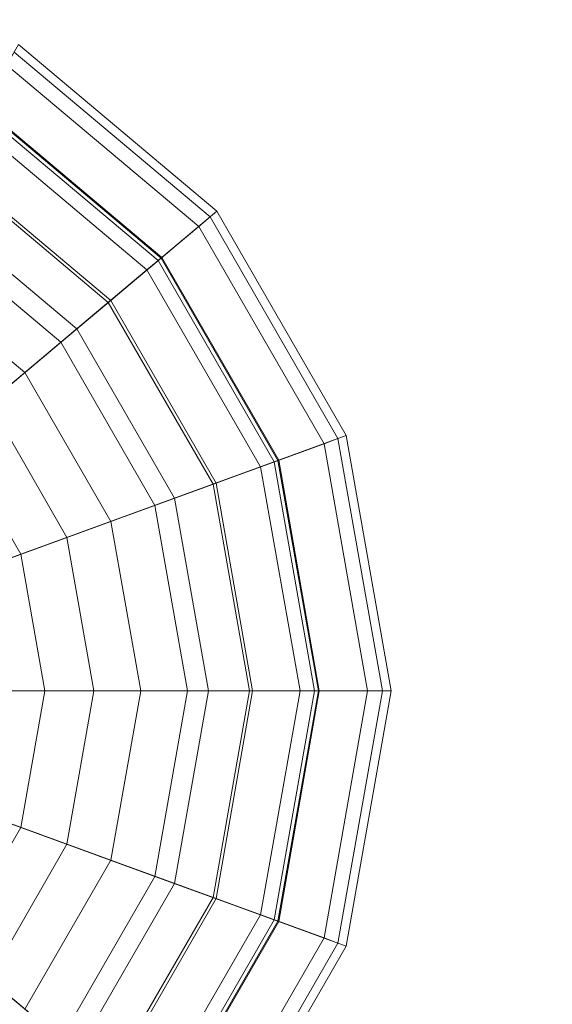
# Model space of a CAD drawing. Units: inches. Extents: x 375 to 1122, y 27 to 1069.
# Tile 100 of 155: x 719.942 to 720.91, y 864.699 to 866.486. Entities that reach past the tile are written whole.
import ezdxf

# ---------------------------------------------------------------- set-up
doc = ezdxf.new("R2010")
doc.units = ezdxf.units.IN
doc.layers.add('A-ANNO-DIMS', color=2, linetype='Continuous', lineweight=18)
doc.layers.add('Furniture', color=30, linetype='Continuous', lineweight=18)
doc.styles.get("Standard").update_dxf_attribs({"font": 'arial.ttf'})
doc.dimstyles.new('ISO-25', dxfattribs={"dimtxt": 12, "dimasz": 2.5, "dimexe": 1.5, "dimexo": 1.5, "dimtad": 1, "dimdec": 1, "dimlunit": 3, "dimtxsty": 'Standard', "dimblk": 'ARCHTICK', "dimcen": 2.5, "dimadec": 0, "dimazin": 0, "dimtfac": 1, "dimtdec": 1, "dimtmove": 0, "dimatfit": 3, "dimfxl": 1.5, "dimfxlon": 1, "dimarcsym": 0})

# ---------------------------------------------------------------- blocks, each defined once
blk = doc.blocks.new('A$C403C54AD')
for points in [[(1.826559, 0.891746, -0.031825), (1.826559, 0.857884, -0.028747), (1.826559, 0.857884, -0.028747), (1.814977, 0.889704, -0.031825)], [(1.826559, 0.88848, -0.028594), (1.826559, 0.891746, -0.031825), (1.814977, 0.889704, -0.031825), (1.816094, 0.886635, -0.028594)], [(1.83814, 0.889704, -0.031825), (1.826559, 0.857884, -0.028747), (1.826559, 0.857884, -0.028747), (1.826559, 0.891746, -0.031825)], [(1.837023, 0.886635, -0.028594), (1.83814, 0.889704, -0.031825), (1.826559, 0.891746, -0.031825), (1.826559, 0.88848, -0.028594)], [(1.826559, 0.88844, 0.131159), (1.826559, 0.891347, 0.117935), (1.815114, 0.889329, 0.117935), (1.816108, 0.886597, 0.131159)], [(1.826559, 0.891347, 0.117935), (1.826559, 0.890672, 0.089693), (1.815345, 0.888695, 0.089693), (1.815114, 0.889329, 0.117935)], [(1.83701, 0.886597, 0.131159), (1.838004, 0.889329, 0.117935), (1.826559, 0.891347, 0.117935), (1.826559, 0.88844, 0.131159)], [(1.838004, 0.889329, 0.117935), (1.837773, 0.888695, 0.089693), (1.826559, 0.890672, 0.089693), (1.826559, 0.891347, 0.117935)], [(1.826559, 0.890672, 0.089693), (1.826559, 0.885308, 0.071684), (1.817179, 0.883654, 0.071684), (1.815345, 0.888695, 0.089693)], [(1.837773, 0.888695, 0.089693), (1.835938, 0.883654, 0.071684), (1.826559, 0.885308, 0.071684), (1.826559, 0.890672, 0.089693)], [(1.816094, 0.886635, -0.028594), (1.814977, 0.889704, -0.031825), (1.804793, 0.883824, -0.031825), (1.806892, 0.881322, -0.028594)], [(1.814977, 0.889704, -0.031825), (1.826559, 0.857884, -0.028747), (1.826559, 0.857884, -0.028747), (1.804793, 0.883824, -0.031825)], [(1.848325, 0.883824, -0.031825), (1.826559, 0.857884, -0.028747), (1.826559, 0.857884, -0.028747), (1.83814, 0.889704, -0.031825)], [(1.846226, 0.881322, -0.028594), (1.848325, 0.883824, -0.031825), (1.83814, 0.889704, -0.031825), (1.837023, 0.886635, -0.028594)], [(1.816108, 0.886597, 0.131159), (1.815114, 0.889329, 0.117935), (1.805049, 0.883518, 0.117935), (1.806918, 0.881291, 0.131159)], [(1.815114, 0.889329, 0.117935), (1.815345, 0.888695, 0.089693), (1.805483, 0.883001, 0.089693), (1.805049, 0.883518, 0.117935)], [(1.8462, 0.881291, 0.131159), (1.848069, 0.883518, 0.117935), (1.838004, 0.889329, 0.117935), (1.83701, 0.886597, 0.131159)], [(1.848069, 0.883518, 0.117935), (1.847635, 0.883001, 0.089693), (1.837773, 0.888695, 0.089693), (1.838004, 0.889329, 0.117935)], [(1.815345, 0.888695, 0.089693), (1.817179, 0.883654, 0.071684), (1.808931, 0.878892, 0.071684), (1.805483, 0.883001, 0.089693)], [(1.826559, 0.872098, -0.02532), (1.826559, 0.88848, -0.028594), (1.816094, 0.886635, -0.028594), (1.821697, 0.871241, -0.02532)], [(1.826559, 0.883444, 0.140564), (1.826559, 0.88844, 0.131159), (1.816108, 0.886597, 0.131159), (1.817817, 0.881902, 0.140564)], [(1.83142, 0.871241, -0.02532), (1.837023, 0.886635, -0.028594), (1.826559, 0.88848, -0.028594), (1.826559, 0.872098, -0.02532)], [(1.835301, 0.881902, 0.140564), (1.83701, 0.886597, 0.131159), (1.826559, 0.88844, 0.131159), (1.826559, 0.883444, 0.140564)], [(1.847635, 0.883001, 0.089693), (1.844187, 0.878892, 0.071684), (1.835938, 0.883654, 0.071684), (1.837773, 0.888695, 0.089693)], [(1.826559, 0.888263, 0.117718), (1.826559, 0.885453, 0.130354), (1.81713, 0.88379, 0.130354), (1.816169, 0.886431, 0.117718)], [(1.826559, 0.887605, 0.090178), (1.826559, 0.888263, 0.117718), (1.816169, 0.886431, 0.117718), (1.816394, 0.885812, 0.090178)], [(1.836949, 0.886431, 0.117718), (1.835988, 0.88379, 0.130354), (1.826559, 0.885453, 0.130354), (1.826559, 0.888263, 0.117718)], [(1.836724, 0.885812, 0.090178), (1.836949, 0.886431, 0.117718), (1.826559, 0.888263, 0.117718), (1.826559, 0.887605, 0.090178)], [(1.826559, 0.882497, 0.073031), (1.826559, 0.887605, 0.090178), (1.816394, 0.885812, 0.090178), (1.818141, 0.881013, 0.073031)], [(1.834977, 0.881013, 0.073031), (1.836724, 0.885812, 0.090178), (1.826559, 0.887605, 0.090178), (1.826559, 0.882497, 0.073031)], [(1.821697, 0.871241, -0.02532), (1.816094, 0.886635, -0.028594), (1.806892, 0.881322, -0.028594), (1.817422, 0.868773, -0.02532)], [(1.817817, 0.881902, 0.140564), (1.816108, 0.886597, 0.131159), (1.806918, 0.881291, 0.131159), (1.81013, 0.877464, 0.140564)], [(1.835696, 0.868773, -0.02532), (1.846226, 0.881322, -0.028594), (1.837023, 0.886635, -0.028594), (1.83142, 0.871241, -0.02532)], [(1.842988, 0.877464, 0.140564), (1.8462, 0.881291, 0.131159), (1.83701, 0.886597, 0.131159), (1.835301, 0.881902, 0.140564)], [(1.816169, 0.886431, 0.117718), (1.81713, 0.88379, 0.130354), (1.808838, 0.879003, 0.130354), (1.807032, 0.881156, 0.117718)], [(1.816394, 0.885812, 0.090178), (1.816169, 0.886431, 0.117718), (1.807032, 0.881156, 0.117718), (1.807455, 0.880651, 0.090178)], [(1.846086, 0.881156, 0.117718), (1.84428, 0.879003, 0.130354), (1.835988, 0.88379, 0.130354), (1.836949, 0.886431, 0.117718)], [(1.845663, 0.880651, 0.090178), (1.846086, 0.881156, 0.117718), (1.836949, 0.886431, 0.117718), (1.836724, 0.885812, 0.090178)], [(1.818141, 0.881013, 0.073031), (1.816394, 0.885812, 0.090178), (1.807455, 0.880651, 0.090178), (1.810738, 0.876739, 0.073031)], [(1.84238, 0.876739, 0.073031), (1.845663, 0.880651, 0.090178), (1.836724, 0.885812, 0.090178), (1.834977, 0.881013, 0.073031)], [(1.826559, 0.885453, 0.130354), (1.826559, 0.880365, 0.140564), (1.81887, 0.879009, 0.140564), (1.81713, 0.88379, 0.130354)], [(1.826559, 0.885308, 0.071684), (1.826559, 0.878242, 0.061451), (1.819596, 0.877014, 0.061451), (1.817179, 0.883654, 0.071684)], [(1.835988, 0.88379, 0.130354), (1.834248, 0.879009, 0.140564), (1.826559, 0.880365, 0.140564), (1.826559, 0.885453, 0.130354)], [(1.835938, 0.883654, 0.071684), (1.833522, 0.877014, 0.061451), (1.826559, 0.878242, 0.061451), (1.826559, 0.885308, 0.071684)], [(1.806892, 0.881322, -0.028594), (1.804793, 0.883824, -0.031825), (1.797233, 0.874815, -0.031825), (1.800062, 0.873182, -0.028594)], [(1.804793, 0.883824, -0.031825), (1.826559, 0.857884, -0.028747), (1.826559, 0.857884, -0.028747), (1.797233, 0.874815, -0.031825)], [(1.855884, 0.874815, -0.031825), (1.826559, 0.857884, -0.028747), (1.826559, 0.857884, -0.028747), (1.848325, 0.883824, -0.031825)], [(1.806918, 0.881291, 0.131159), (1.805049, 0.883518, 0.117935), (1.797579, 0.874616, 0.117935), (1.800097, 0.873162, 0.131159)], [(1.805049, 0.883518, 0.117935), (1.805483, 0.883001, 0.089693), (1.798163, 0.874278, 0.089693), (1.797579, 0.874616, 0.117935)], [(1.81713, 0.88379, 0.130354), (1.81887, 0.879009, 0.140564), (1.812108, 0.875106, 0.140564), (1.808838, 0.879003, 0.130354)], [(1.817179, 0.883654, 0.071684), (1.819596, 0.877014, 0.061451), (1.813473, 0.873479, 0.061451), (1.808931, 0.878892, 0.071684)], [(1.826559, 0.880365, 0.140564), (1.826559, 0.883444, 0.140564), (1.817817, 0.881902, 0.140564), (1.81887, 0.879009, 0.140564)], [(1.834248, 0.879009, 0.140564), (1.835301, 0.881902, 0.140564), (1.826559, 0.883444, 0.140564), (1.826559, 0.880365, 0.140564)], [(1.844187, 0.878892, 0.071684), (1.839644, 0.873479, 0.061451), (1.833522, 0.877014, 0.061451), (1.835938, 0.883654, 0.071684)], [(1.84428, 0.879003, 0.130354), (1.84101, 0.875106, 0.140564), (1.834248, 0.879009, 0.140564), (1.835988, 0.88379, 0.130354)], [(1.805483, 0.883001, 0.089693), (1.808931, 0.878892, 0.071684), (1.802809, 0.871596, 0.071684), (1.798163, 0.874278, 0.089693)], [(1.826559, 0.876011, 0.063639), (1.826559, 0.882497, 0.073031), (1.818141, 0.881013, 0.073031), (1.820359, 0.874918, 0.063639)], [(1.832759, 0.874918, 0.063639), (1.834977, 0.881013, 0.073031), (1.826559, 0.882497, 0.073031), (1.826559, 0.876011, 0.063639)], [(1.81887, 0.879009, 0.140564), (1.817817, 0.881902, 0.140564), (1.81013, 0.877464, 0.140564), (1.812108, 0.875106, 0.140564)], [(1.84101, 0.875106, 0.140564), (1.842988, 0.877464, 0.140564), (1.835301, 0.881902, 0.140564), (1.834248, 0.879009, 0.140564)], [(1.817422, 0.868773, -0.02532), (1.806892, 0.881322, -0.028594), (1.800062, 0.873182, -0.028594), (1.814249, 0.864991, -0.02532)], [(1.81013, 0.877464, 0.140564), (1.806918, 0.881291, 0.131159), (1.800097, 0.873162, 0.131159), (1.804424, 0.870664, 0.140564)], [(1.807032, 0.881156, 0.117718), (1.808838, 0.879003, 0.130354), (1.802683, 0.871669, 0.130354), (1.80025, 0.873073, 0.117718)], [(1.807455, 0.880651, 0.090178), (1.807032, 0.881156, 0.117718), (1.80025, 0.873073, 0.117718), (1.80082, 0.872744, 0.090178)], [(1.838869, 0.864991, -0.02532), (1.853056, 0.873182, -0.028594), (1.846226, 0.881322, -0.028594), (1.835696, 0.868773, -0.02532)], [(1.820359, 0.874918, 0.063639), (1.818141, 0.881013, 0.073031), (1.810738, 0.876739, 0.073031), (1.814907, 0.87177, 0.063639)], [(1.838211, 0.87177, 0.063639), (1.84238, 0.876739, 0.073031), (1.834977, 0.881013, 0.073031), (1.832759, 0.874918, 0.063639)], [(1.810738, 0.876739, 0.073031), (1.807455, 0.880651, 0.090178), (1.80082, 0.872744, 0.090178), (1.805243, 0.87019, 0.073031)], [(1.808838, 0.879003, 0.130354), (1.812108, 0.875106, 0.140564), (1.80709, 0.869125, 0.140564), (1.802683, 0.871669, 0.130354)], [(1.808931, 0.878892, 0.071684), (1.813473, 0.873479, 0.061451), (1.808929, 0.868063, 0.061451), (1.802809, 0.871596, 0.071684)], [(1.850309, 0.871596, 0.071684), (1.844189, 0.868063, 0.061451), (1.839644, 0.873479, 0.061451), (1.844187, 0.878892, 0.071684)], [(1.826559, 0.878242, 0.061451), (1.826559, 0.868003, 0.054084), (1.823098, 0.867392, 0.054084), (1.819596, 0.877014, 0.061451)], [(1.833522, 0.877014, 0.061451), (1.83002, 0.867392, 0.054084), (1.826559, 0.868003, 0.054084), (1.826559, 0.878242, 0.061451)], [(1.812108, 0.875106, 0.140564), (1.81013, 0.877464, 0.140564), (1.804424, 0.870664, 0.140564), (1.80709, 0.869125, 0.140564)], [(1.814907, 0.87177, 0.063639), (1.810738, 0.876739, 0.073031), (1.805243, 0.87019, 0.073031), (1.81086, 0.866948, 0.063639)], [(1.819596, 0.877014, 0.061451), (1.823098, 0.867392, 0.054084), (1.820055, 0.865635, 0.054084), (1.813473, 0.873479, 0.061451)], [(1.839644, 0.873479, 0.061451), (1.833063, 0.865635, 0.054084), (1.83002, 0.867392, 0.054084), (1.833522, 0.877014, 0.061451)], [(1.842258, 0.866948, 0.063639), (1.847874, 0.87019, 0.073031), (1.84238, 0.876739, 0.073031), (1.838211, 0.87177, 0.063639)], [(1.826559, 0.866788, 0.057003), (1.826559, 0.876011, 0.063639), (1.820359, 0.874918, 0.063639), (1.823514, 0.866251, 0.057003)], [(1.829604, 0.866251, 0.057003), (1.832759, 0.874918, 0.063639), (1.826559, 0.876011, 0.063639), (1.826559, 0.866788, 0.057003)], [(1.823514, 0.866251, 0.057003), (1.820359, 0.874918, 0.063639), (1.814907, 0.87177, 0.063639), (1.820835, 0.864705, 0.057003)], [(1.832282, 0.864705, 0.057003), (1.838211, 0.87177, 0.063639), (1.832759, 0.874918, 0.063639), (1.829604, 0.866251, 0.057003)]]:
    blk.add_3dface(points)
blk = doc.blocks.new('_ArchTick')
at = {"color": 0, "linetype": 'ByBlock', "const_width": 0.15}
blk.add_lwpolyline([(-0.5, -0.5), (0.5, 0.5)], dxfattribs=at)
blk = doc.blocks.new('*D85')
at = {"layer": 'A-ANNO-DIMS', "color": 0, "lineweight": -2, "transparency": 16777216}
for p, q in [((401.5073, 868.5277), (398.5073, 868.5277)), ((400.0073, 814.5277), (400.0073, 868.5277)), ((401.5073, 814.5277), (398.5073, 814.5277))]:
    blk.add_line(p, q, dxfattribs=at)
at = {"layer": 'Defpoints', "color": 0, "transparency": 16777216}
for p in [(400.0073, 868.5277), (845.0073, 868.5277), (845.0073, 814.5277)]:
    blk.add_point(p, dxfattribs=at)
at = {"layer": 'A-ANNO-DIMS', "color": 0, "lineweight": -2, "transparency": 16777216, "xscale": 2.5, "yscale": 2.5, "zscale": 2.5}
for p, rotation in [((400.0073, 868.5277), 90), ((400.0073, 814.5277), 270)]:
    blk.add_blockref('_ArchTick', p, dxfattribs=dict(at, rotation=rotation))
at = {"layer": 'A-ANNO-DIMS', "color": 0, "transparency": 16777216, "insert": (393.2555, 841.5277), "char_height": 12, "attachment_point": 5, "rotation": 90}
blk.add_mtext('4\'-6"', dxfattribs=at)

msp = doc.modelspace()

# ---------------------------------------------------------------- block references
at = {"layer": 'Furniture', "xscale": 39.9918517141215, "yscale": 39.9918517141215, "zscale": 39.9918517141215, "rotation": 270}
msp.add_blockref('A$C403C54AD', (684.9549, 938.3156, 0.024), dxfattribs=at)

# ---------------------------------------------------------------- dimensions: what is measured, and where the dimension line sits
at = {"layer": 'A-ANNO-DIMS'}
dim = msp.add_linear_dim(base=(400.0073, 868.5277), p1=(845.0073, 814.5277), p2=(845.0073, 868.5277), angle=90, dimstyle='ISO-25', override={"dimdec": 1, "dimlfac": 1, "dimrnd": 0, "dimzin": 1, "dimdsep": 46, "dimlunit": 4, "dimfrac": 2}, dxfattribs=at)
dim.commit()
dim.dimension.update_dxf_attribs({"geometry": '*D85', "text_midpoint": (393.2555, 841.5277)})

doc.saveas('drawing.dxf')
